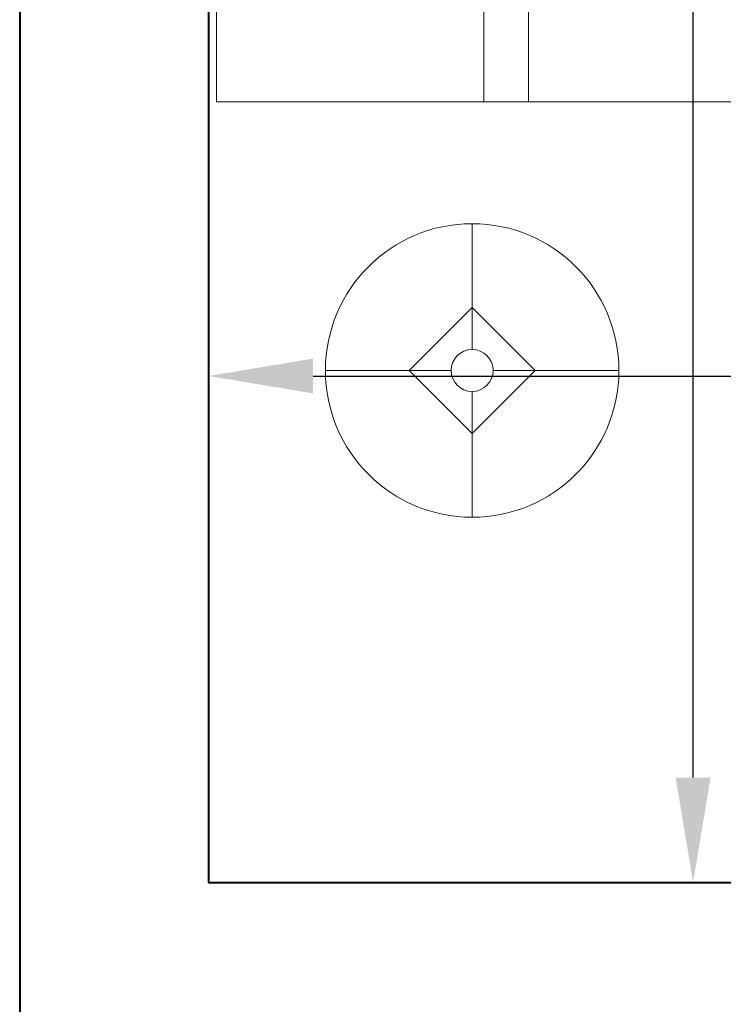
# Model space of a CAD drawing. Units: inches. Extents: x -301 to 715, y -607 to 364.
# Tile 68 of 141: x -205 to -171, y -73 to -26. Entities that reach past the tile are written whole.
import ezdxf

# ---------------------------------------------------------------- set-up
doc = ezdxf.new("R2010")
doc.units = ezdxf.units.IN
doc.header["$MEASUREMENT"] = 0
for name, color, linetype, lineweight in [('A-ANNO-DIMS', 2, 'Continuous', 18), ('A-FURN', 8, 'Continuous', 18), ('A-WALL', 3, 'Continuous', 40)]:
    doc.layers.add(name, color=color, linetype=linetype, lineweight=lineweight)
doc.styles.get("Standard").update_dxf_attribs({"font": 'arial.ttf'})
doc.dimstyles.get("Standard").update_dxf_attribs({"dimtxt": 0.18, "dimasz": 0.18, "dimexe": 0.18, "dimexo": 0.0625, "dimgap": 0.09, "dimtad": 0, "dimtih": 1, "dimtoh": 1, "dimdec": 1, "dimzin": 0, "dimdsep": 46, "dimlunit": 4, "dimtxsty": 'Standard', "dimcen": 0.09, "dimclrd": 3, "dimclre": 4, "dimclrt": 6, "dimadec": 0, "dimazin": 0, "dimtfac": 1, "dimtdec": 1, "dimtofl": 0, "dimtmove": 0, "dimatfit": 3, "dimfxl": 1, "dimtfill": 2, "dimtfillclr": 51, "dimtolj": 1, "dimtzin": 0, "dimarcsym": 0})

# ---------------------------------------------------------------- blocks, each defined once
blk = doc.blocks.new('Bed - Queen')
for p, q in [((0, -80.00003), (0, 0)), ((0, 0), (59.99999, 0)), ((0, -14.4), (44.8, -14.4)), ((44.8, -16.8), (0, -16.8))]:
    blk.add_line(p, q)
blk = doc.blocks.new('Lamp - Table')
for p, q in [((0, 7), (0, 1)), ((0, 3), (-3, 0)), ((3, 0), (0, 3)), ((-1, 0), (-7, 0)), ((-3, 0), (0, -3)), ((0, -3), (3, 0)), ((1, 0), (7, 0)), ((0, -1), (0, -7))]:
    blk.add_line(p, q)
for radius in [7, 1]:
    blk.add_circle((0, 0), radius)
blk = doc.blocks.new('*D56')
at = {"layer": 'A-ANNO-DIMS', "color": 0, "lineweight": -2, "transparency": 16777216}
for p, q in [((-195.541, 65.682), (-172.295, 65.682)), ((-172.475, 60.682), (-172.475, 0.778)), ((-172.475, -62.318), (-172.475, -2.414)), ((-195.541, -67.318), (-172.295, -67.318))]:
    blk.add_line(p, q, dxfattribs=at)
at = {"layer": 'A-ANNO-DIMS', "color": 0, "transparency": 16777216}
for points in [[(-173.308, 60.682), (-171.641, 60.682), (-172.475, 65.682)], [(-173.308, -62.318), (-171.641, -62.318), (-172.475, -67.318)]]:
    blk.add_solid(points, dxfattribs=at)
at = {"layer": 'Defpoints', "color": 0, "transparency": 16777216}
for p in [(-195.603, 65.682), (-172.475, 65.682), (-195.603, -67.318)]:
    blk.add_point(p, dxfattribs=at)
at = {"layer": 'A-ANNO-DIMS', "color": 0, "transparency": 16777216, "insert": (-172.475, -0.818), "char_height": 3, "attachment_point": 5, "bg_fill": 1, "box_fill_scale": 1.25, "bg_fill_color": 51, "bg_fill_transparency": 0}
blk.add_mtext('\\A1;11\'-1"', dxfattribs=at)
blk = doc.blocks.new('*D57')
at = {"layer": 'A-ANNO-DIMS', "color": 0, "lineweight": -2, "transparency": 16777216}
for p, q in [((-195.603, -67.255), (-195.603, -42.99)), ((-190.603, -43.17), (-126.098, -43.17)), ((-56.603, -43.17), (-121.109, -43.17)), ((-51.603, -67.255), (-51.603, -42.99))]:
    blk.add_line(p, q, dxfattribs=at)
at = {"layer": 'A-ANNO-DIMS', "color": 0, "transparency": 16777216}
for points in [[(-190.603, -42.336), (-190.603, -44.003), (-195.603, -43.17)], [(-56.603, -42.336), (-56.603, -44.003), (-51.603, -43.17)]]:
    blk.add_solid(points, dxfattribs=at)
at = {"layer": 'Defpoints', "color": 0, "transparency": 16777216}
for p in [(-51.603, -43.17), (-195.603, -67.318), (-51.603, -67.318)]:
    blk.add_point(p, dxfattribs=at)
at = {"layer": 'A-ANNO-DIMS', "color": 0, "transparency": 16777216, "insert": (-123.603, -43.17), "char_height": 3, "attachment_point": 5, "bg_fill": 1, "box_fill_scale": 1.25, "bg_fill_color": 51, "bg_fill_transparency": 0}
blk.add_mtext("\\A1;12'", dxfattribs=at)
blk = doc.blocks.new('*D151')
at = {"layer": 'A-ANNO-DIMS', "color": 4, "lineweight": -2, "transparency": 16777216}
for p, q in [((-204.603, -223.755), (-204.603, 359.612)), ((-45.603, -214.755), (-45.603, 359.612))]:
    blk.add_line(p, q, dxfattribs=at)
at = {"layer": 'A-ANNO-DIMS', "color": 3, "lineweight": -2, "transparency": 16777216}
for p, q in [((-204.423, 359.432), (-125.494, 359.432)), ((-45.783, 359.432), (-124.713, 359.432))]:
    blk.add_line(p, q, dxfattribs=at)
at = {"layer": 'A-ANNO-DIMS', "color": 3, "transparency": 16777216}
for points in [[(-204.423, 359.462), (-204.423, 359.402), (-204.603, 359.432)], [(-45.783, 359.462), (-45.783, 359.402), (-45.603, 359.432)]]:
    blk.add_solid(points, dxfattribs=at)
at = {"layer": 'Defpoints', "color": 0, "transparency": 16777216}
for p in [(-45.603, 359.432), (-45.603, -214.818), (-204.603, -223.818)]:
    blk.add_point(p, dxfattribs=at)
at = {"layer": 'A-ANNO-DIMS', "color": 6, "transparency": 16777216, "insert": (-125.103, 359.432), "char_height": 0.18, "attachment_point": 5, "bg_fill": 1, "box_fill_scale": 1.25, "bg_fill_color": 51, "bg_fill_transparency": 0}
blk.add_mtext('\\A1;13\'-3"', dxfattribs=at)

msp = doc.modelspace()

# ---------------------------------------------------------------- linework, layer by layer
at = {"layer": 'A-WALL'}
for p, q in [((-204.603, 71.682), (-204.603, -67.318)), ((-195.603, 65.682), (-195.603, -67.318)), ((-204.603, -67.318), (-204.603, -223.818)), ((-195.603, -67.318), (-51.603, -67.318))]:
    msp.add_line(p, q, dxfattribs=at)

# ---------------------------------------------------------------- block references
at = {"layer": 'A-FURN', "xscale": 0.8856750462000775, "yscale": 0.8856750462000775, "zscale": 0.8856750462000775, "rotation": 90}
msp.add_blockref('Bed - Queen', (-195.207, -30.095), dxfattribs=at)
at = {"layer": 'A-FURN'}
msp.add_blockref('Lamp - Table', (-183.017, -42.906), dxfattribs=at)

# ---------------------------------------------------------------- dimensions: what is measured, and where the dimension line sits
at = {"layer": 'A-ANNO-DIMS'}
for base, p1, p2, override, picture, middle in [((-45.603, 359.432), (-204.603, -223.818), (-45.603, -214.818), {"dimdec": 1, "dimlfac": 1, "dimrnd": 0, "dimzin": 1, "dimdsep": 46, "dimlunit": 4, "dimfrac": 2}, '*D151', (-125.103, 359.432)), ((-51.603, -43.17), (-195.603, -67.318), (-51.603, -67.318), {"dimtxt": 3, "dimasz": 5, "dimclrd": 0, "dimclre": 0, "dimclrt": 0}, '*D57', (-123.603, -43.17))]:
    dim = msp.add_linear_dim(base=base, p1=p1, p2=p2, dimstyle='Standard', override=override, dxfattribs=at)
    dim.commit()
    dim.dimension.update_dxf_attribs({"geometry": picture, "text_midpoint": middle})
dim = msp.add_linear_dim(base=(-172.475, 65.682), p1=(-195.603, -67.318), p2=(-195.603, 65.682), angle=90, dimstyle='Standard', override={"dimtxt": 3, "dimasz": 5, "dimclrd": 0, "dimclre": 0, "dimclrt": 0}, dxfattribs=at)
dim.commit()
dim.dimension.update_dxf_attribs({"geometry": '*D56', "text_midpoint": (-172.475, -0.818)})

doc.saveas('drawing.dxf')
